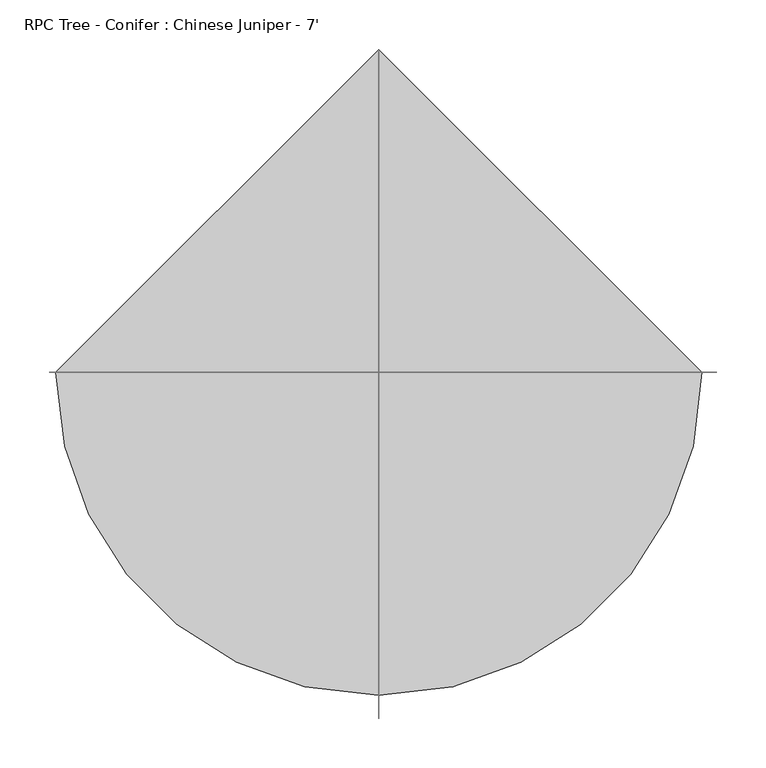
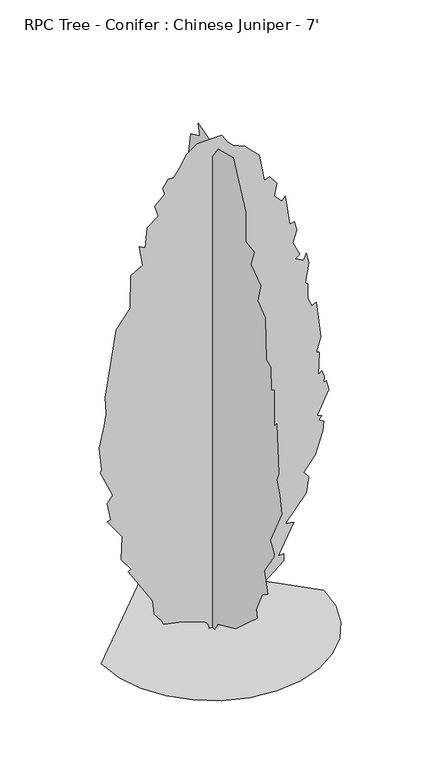
"""IFC4 building model written with IfcOpenShell, lengths in millimetres: geographic element geometry, RPC Tree - Conifer : Chinese Juniper - 7'."""

from ifc_helpers import new_model, si_unit, origin, place, context, project, spatial, triangles, source, transform, mapped, element, save


def rpc_tree_conifer_chinese_juniper_7_7598bbdc(model_context):
    return source(origin(), model_context, "Body", "Tessellation", [
        triangles([(-10.3135556, 5e-07, 9e-07), (-12.8060293, -2e-07, 12.8140684), (-19.5312093, -4e-07, 21.7081794), (-88.2070433, 1.1e-06, 46.9827109), (-143.9981418, 2.8e-06, 58.8213279), (-149.3455807, 2.2e-06, 72.1897524), (-170.8912042, 1.5e-06, 99.7706089), (-176.0828022, -7e-07, 141.7057854), (-184.1045146, -1.3e-06, 157.7479294), (-248.2723821, -4.6e-06, 259.3475236), (-239.9701817, -5.3e-06, 264.3368267), (-268.362017, -6.4e-06, 304.1387577), (-265.4845582, -1.07e-05, 374.7346484), (-309.7677564, -1.24e-05, 435.812788), (-299.0725335, -1.31e-05, 438.4852266), (-309.3523021, -1.58e-05, 492.5148502), (-293.7240046, -1.78e-05, 513.3483533), (-331.1564581, -2.11e-05, 596.2342461), (-325.8097278, -2.16e-05, 601.5809764), (-333.8307135, -2.56e-05, 673.7698477), (-319.3200076, -2.99e-05, 736.7529219), (-312.4402313, -3.24e-05, 772.6976755), (-315.1144867, -3.53e-05, 823.4978451), (-283.0305802, -4.87e-05, 1024.024268), (-242.9256517, -5.36e-05, 1077.4986929), (-240.7575791, -5.96e-05, 1177.3046648), (-205.4931982, -6.24e-05, 1197.8151861), (-216.1884393, -6.56e-05, 1259.3087437), (-197.9348478, -6.58e-05, 1248.8367085), (-192.1255003, -6.97e-05, 1310.1089859), (-160.0402858, -7.25e-05, 1334.1719067), (-170.7351817, -7.41e-05, 1368.9301048), (-141.3244133, -7.7e-05, 1395.667281), (-146.6718613, -7.79e-05, 1414.3835804), (-130.6297082, -8e-05, 1438.4465012), (-114.5875642, -8.07e-05, 1438.4465012), (-96.1815747, -8.29e-05, 1462.3443157), (-77.7287857, -8.58e-05, 1497.0336227), (-44.6214088, -8.86e-05, 1519.4527485), (26.5664902, -9.18e-05, 1520.5723022), (43.1603652, -9.1e-05, 1494.5933647), (59.2025137, -9.07e-05, 1478.551466), (94.8687642, -9.14e-05, 1463.445702), (136.7395278, -9.06e-05, 1419.7303471), (152.7816628, -8.64e-05, 1336.846162), (168.8238158, -8.74e-05, 1342.1929287), (188.3895002, -8.66e-05, 1314.20205), (182.191877, -8.41e-05, 1278.0250431), (203.5823773, -8.36e-05, 1253.9621223), (214.2758017, -8.47e-05, 1264.6573997), (227.6453163, -7.99e-05, 1173.7504486), (241.0130141, -8.06e-05, 1176.424704), (248.2828829, -7.94e-05, 1149.9378759), (236.3339574, -7.67e-05, 1113.592202), (257.0549855, -7.5e-05, 1069.4776709), (243.0450304, -7.39e-05, 1061.0775295), (267.7502266, -7.42e-05, 1048.0871887), (275.7712123, -7.56e-05, 1066.8034155), (283.792198, -7.41e-05, 1034.7194727), (273.0987737, -7.01e-05, 975.8983538), (280.8185786, -7.01e-05, 969.5464886), (279.746333, -6.74e-05, 926.116), (291.8131837, -6.63e-05, 898.3609354), (305.1827165, -6.72e-05, 903.7077021), (318.5503962, -6.11e-05, 791.4139023), (305.1827165, -5.8e-05, 748.6347548), (313.5084801, -5.81e-05, 745.8062937), (310.5294468, -5.39e-05, 676.4441031), (321.2246879, -5.48e-05, 684.4650524), (329.2456736, -5.41e-05, 665.7488256), (326.5713819, -5.28e-05, 647.0344156), (334.5923676, -5.33e-05, 649.7068542), (342.6133533, -5.19e-05, 620.2971668), (307.8551551, -4.63e-05, 550.7808068), (321.2246879, -4.65e-05, 545.4340765), (313.2037022, -4.56e-05, 534.7388354), (326.5713819, -4.57e-05, 526.7178497), (323.7592352, -4.38e-05, 497.9014764), (302.5084248, -3.89e-05, 430.4642409), (267.7502266, -3.48e-05, 387.6850571), (283.792198, -3.44e-05, 368.9688303), (275.0237288, -3.12e-05, 322.2617249), (214.2758017, -2.4e-05, 245.9798258), (238.3405755, -2.49e-05, 243.3055704), (192.8871181, -1.77e-05, 155.0742009), (208.9290895, -1.84e-05, 155.0742009), (208.9290895, -1.71e-05, 133.684618), (91.2864429, -6.2e-06, 37.4317359), (91.2864429, -7e-06, 50.8001605), (11.0759977, -5e-07, 0.0), (0.1966718, 9.8494079, 9.29e-05), (0.1966729, 24.6293697, 10.2116678), (0.1966747, 55.3021477, 21.3897713), (0.1966762, 127.4919001, 48.1266227), (0.1966794, 164.923636, 82.8846392), (0.1966788, 148.881492, 85.5583586), (0.1966849, 206.1035171, 168.0404152), (0.1966859, 188.9874833, 208.5473722), (0.1966882, 237.1133793, 278.0637686), (0.1966893, 231.7666672, 310.147675), (0.1966927, 266.5230486, 352.9268589), (0.1966955, 278.2089087, 404.0935395), (0.1966947, 271.8715775, 457.2014534), (0.1966993, 314.6507795, 521.369339), (0.1967023, 317.3232182, 585.539005), (0.1967039, 301.8799747, 638.0518244), (0.1967057, 325.3442039, 721.897506), (0.1967061, 303.9555203, 751.3071934), (0.1967086, 277.2183078, 836.8655611), (0.1967091, 295.9345346, 895.68668), (0.1967119, 274.5440343, 981.2450478), (0.196713, 247.8086386, 1032.0452173), (0.1967142, 234.439124, 1138.9940672), (0.1967132, 218.3971526, 1130.9731178), (0.1967174, 218.3971526, 1227.2249462), (0.1967163, 186.3132279, 1235.2458229), (0.1967152, 169.3394457, 1292.3597786), (0.1967168, 159.5761971, 1339.5204174), (0.1967168, 127.4919001, 1371.6043602), (0.1967204, 111.449747, 1467.8579327), (0.1967164, 65.9968483, 1489.2467434), (0.1967182, 72.8998653, 1523.6638287), (0.1967145, 8.1062543, 1503.0081127), (0.1967152, 4.5019648, 1457.1628006), (0.1967129, -27.5823121, 1502.6161308), (0.1967105, -105.1193285, 1524.0049416), (0.1967048, -169.2880862, 1392.9930256), (0.1967008, -169.2880862, 1302.0879639), (0.1966987, -211.5754214, 1294.5605164), (0.1966973, -193.3508616, 1245.9411003), (0.1966964, -244.8876323, 1210.7601809), (0.1966946, -230.7833333, 1155.0360386), (0.1966917, -268.2139701, 1125.6245344), (0.1966887, -273.562499, 997.2870192), (0.1966873, -295.3920532, 987.9742882), (0.1966841, -297.6254561, 917.0771622), (0.1966839, -313.6674093, 927.7706228), (0.1966819, -313.6674093, 815.4768957), (0.1966791, -327.0351254, 831.5188671), (0.196675, -337.7303664, 681.7926138), (0.1966744, -326.120719, 656.3254183), (0.1966719, -343.0789135, 617.6229115), (0.1966721, -351.0998629, 564.1485229), (0.1966695, -294.9511826, 449.1804677), (0.1966673, -313.6674093, 417.0965612), (0.1966698, -312.0853475, 405.769927), (0.1966688, -262.8672579, 334.2124489), (0.1966653, -281.5834847, 272.7170382), (0.1966657, -252.1719987, 254.0008115), (0.1966671, -222.7623476, 189.8329441), (0.1966658, -228.1090598, 165.7690968), (0.196666, -174.6353615, 117.6426557), (0.1966663, -118.4877531, 66.8424907), (0.1966685, -24.9082271, 24.0633114), (0.1966709, -11.5401454, 9.16e-05), (-327.063394, 0.0, 0.0001066), (-318.4110515, -74.9863023, 0.0001017), (-293.7711855, -143.8493682, 9.65e-05), (-255.1158779, -204.615799, 9.12e-05), (-204.4191359, -255.312541, 8.6e-05), (-143.652696, -293.9678487, 8.1e-05), (-74.7896301, -318.6077328, 7.66e-05), (0.1966858, -327.2600753, 7.28e-05), (75.1829745, -318.6077328, 7e-05), (144.0460404, -293.9678487, 6.85e-05), (204.8124621, -255.312541, 6.81e-05), (255.5092041, -204.615799, 6.89e-05), (294.1645118, -143.8491865, 7.08e-05), (318.8044141, -74.9863023, 7.39e-05), (327.4567566, 2.86e-05, 7.8e-05), (0.1966283, 327.2600753, 0.0001118)], [[57, 58, 59], [27, 28, 29], [87, 88, 89], [49, 50, 51], [13, 14, 15], [83, 84, 85], [74, 75, 76], [63, 64, 65], [68, 69, 70], [71, 72, 73], [9, 10, 11], [85, 86, 87], [85, 87, 89], [51, 52, 53], [54, 55, 56], [90, 1, 2], [66, 67, 68], [45, 46, 47], [17, 18, 19], [68, 70, 71], [45, 47, 48], [31, 32, 33], [76, 77, 78], [89, 90, 2], [89, 2, 3], [57, 59, 60], [51, 53, 54], [25, 26, 27], [39, 40, 41], [56, 57, 60], [71, 73, 74], [34, 35, 36], [33, 34, 36], [4, 5, 6], [60, 61, 62], [80, 81, 82], [38, 39, 41], [37, 38, 41], [37, 41, 42], [29, 30, 31], [15, 16, 17], [36, 37, 42], [33, 36, 42], [31, 33, 42], [31, 42, 43], [31, 43, 44], [31, 44, 45], [29, 31, 45], [29, 45, 48], [27, 29, 48], [25, 27, 48], [25, 48, 49], [25, 49, 51], [25, 51, 54], [25, 54, 56], [25, 56, 60], [25, 60, 62], [24, 25, 62], [23, 24, 62], [22, 23, 62], [22, 62, 63], [22, 63, 65], [22, 65, 66], [22, 66, 68], [21, 22, 68], [20, 21, 68], [19, 20, 68], [17, 19, 68], [17, 68, 71], [17, 71, 74], [15, 17, 74], [13, 15, 74], [13, 74, 76], [13, 76, 78], [13, 78, 79], [13, 79, 80], [12, 13, 80], [11, 12, 80], [9, 11, 80], [9, 80, 82], [9, 82, 83], [9, 83, 85], [9, 85, 89], [9, 89, 3], [9, 3, 4], [8, 9, 4], [8, 4, 6], [7, 8, 6], [138, 139, 140], [94, 95, 96], [136, 137, 138], [121, 122, 123], [112, 113, 114], [128, 129, 130], [121, 123, 124], [125, 126, 127], [124, 125, 127], [114, 115, 116], [147, 148, 149], [130, 131, 132], [124, 127, 128], [134, 135, 136], [154, 155, 91], [154, 91, 92], [150, 151, 152], [96, 97, 98], [119, 120, 121], [119, 121, 124], [119, 124, 128], [118, 119, 128], [117, 118, 128], [116, 117, 128], [116, 128, 130], [114, 116, 130], [114, 130, 132], [112, 114, 132], [112, 132, 133], [112, 133, 134], [112, 134, 136], [111, 112, 136], [110, 111, 136], [109, 110, 136], [109, 136, 138], [109, 138, 140], [109, 140, 141], [108, 109, 141], [107, 108, 141], [106, 107, 141], [105, 106, 141], [104, 105, 141], [103, 104, 141], [103, 141, 142], [103, 142, 143], [103, 143, 144], [102, 103, 144], [101, 102, 144], [100, 101, 144], [100, 144, 145], [100, 145, 146], [100, 146, 147], [100, 147, 149], [100, 149, 150], [100, 150, 152], [100, 152, 153], [100, 153, 154], [99, 100, 154], [98, 99, 154], [96, 98, 154], [96, 154, 92], [96, 92, 93], [96, 93, 94], [170, 171, 156], [169, 170, 156], [169, 156, 157], [168, 169, 157], [168, 157, 158], [168, 158, 159], [167, 168, 159], [166, 167, 159], [166, 159, 160], [166, 160, 161], [166, 161, 162], [166, 162, 163], [166, 163, 164], [166, 164, 165]], closed=False),
    ])


if __name__ == "__main__":
    model = new_model("IFC4")
    model_context = context("Model", 3, world=origin())
    ifc_project = project(units=[si_unit("LENGTHUNIT", "METRE", prefix="MILLI")], contexts=[model_context])
    site = spatial("IfcSite", under=ifc_project)
    building = spatial("IfcBuilding", under=site)
    placement = place(None, origin())
    rpc_tree_conifer_chinese_juniper_7_shape = rpc_tree_conifer_chinese_juniper_7_7598bbdc(model_context)
    element("IfcGeographicElement", 1, ObjectType="RPC Tree - Conifer : Chinese Juniper - 7'", at=placement, inside=building, context=model_context, shape_type="MappedRepresentation", body=[
        mapped(rpc_tree_conifer_chinese_juniper_7_shape, transform((0.0, 0.0, 0.0), x_axis=(1.0, 0.0, 0.0), y_axis=(0.0, 1.0, 0.0), z_axis=(0.0, 0.0, 1.0))),
    ])
    save(model, "model.ifc")

# Revit data of these elements
# Type "RPC Tree - Conifer : Chinese Juniper - 7'"
#   built-in parameter 1005198 = "{2, 15},{39, RPC-16-FUM3-UUQ0-UBF0-N000-ST1L-LVER-AU},{1, 0},{1, 0},{2, 35},{1, 8},{5, Color},{1, 0},{1, 0},{3, 0.8},{3, 0.8},{3, 0.8},{1, 8},{7, BBoxMin},{1, 0},{1, 0},{1, 0},{1, 0},{1, 0},{1, 8},{7, BBoxMax},{1, 0},{1, 0},{1, 0},{1, 0},{1, 0},{2, 11},{9, RPCTypeId},{1, 0},{1, 0},{39, RPC-16-FUM3-UUQ0-UBF0-N000-ST1L-LVER-AU},{1, 6},{14, RPCPlantHeight},{1, 0},{1, 0},{1, 7},{2, 11},{7, keyword},{1, 0},{1, 0},{96, :Geometry:RPC:Chinese Juniper:juniperus chinensis:chinese:juniper:cupressaceae:conifer:evergreen},{2, 11},{8, category},{1, 0},{1, 0},{16, :Trees [General]},{2, 11},{12, LocalizedUID},{1, 0},{1, 0},{15, Chinese Juniper},{2, 14},{6, Height},{1, 0},{1, 0},{1, 7},{1, 2},{16, Cast Reflections},{1, 0},{1, 0},{1, 0},{1, 2},{12, Cast Shadows},{1, 0},{1, 0},{1, 1},{1, 2},{9, Lock View},{1, 0},{1, 0},{1, 0},{1, 4},{5, ViewC},{1, 0},{1, 0},{1, 0},{2, 11},{20, AdvancedUIDefinition},{1, 0},{1, 0},{0, },{2, 11},{10, AssetLibID},{1, 0},{1, 0},{36, 4D3F6E72-3F99-4203-98E9-AF80B3C7A7A4},{2, 11},{10, BaseSchema},{1, 0},{1, 0},{9, RPCSchema},{2, 11},{12, ExchangeGUID},{1, 0},{1, 0},{0, },{1, 2},{6, Hidden},{1, 0},{1, 0},{1, 0},{1, 4},{11, RPCCategory},{1, 0},{1, 0},{1, 0},{2, 11},{8, RPCImage},{1, 0},{1, 0},{0, },{1, 4},{13, SchemaVersion},{1, 0},{1, 0},{1, 4},{2, 11},{12, UIDefinition},{1, 0},{1, 0},{0, },{2, 11},{6, UIName},{1, 0},{1, 0},{39, RPC-16-FUM3-UUQ0-UBF0-N000-ST1L-LVER-AU},{2, 11},{11, VersionGUID},{1, 0},{1, 0},{9, RPCSchema},{2, 11},{9, assettype},{1, 0},{1, 0},{11, RPCGeometry},{2, 11},{11, description},{1, 0},{1, 0},{0, },{2, 11},{9, localname},{1, 0},{1, 0},{3, RPC},{2, 11},{9, localtype},{1, 0},{1, 0},{3, RPC},{1, 4},{8, revision},{1, 0},{1, 0},{1, 1},{2, 11},{9, thumbnail},{1, 0},{1, 0},{0, },{1, 4},{7, version},{1, 0},{1, 0},{1, 1},{1, 2},{20, RPC_Cast Reflections},{1, 0},{1, 0},{1, 1},{1, 2},{16, RPC_Cast Shadows},{1, 0},{1, 0},{1, 1},{1, 2},{13, RPC_Lock View},{1, 0},{1, 0},{1, 0},{1, 4},{9, RPC_ViewC},{1, 0},{1, 0},{1, 0},{21, assetlibrary_base.fbx},{1, 5},"
#   built-in parameter 1005195 = "RPC-16-FUM3-UUQ0-UBF0-N000-ST1L-LVER-AU"
#   Type Comments = "Chinese Juniper"
#   Assembly Code = "G2050500"
#   Height = 5' - 0"
#   Description = (empty or 0)
#   Default Elevation = 0
